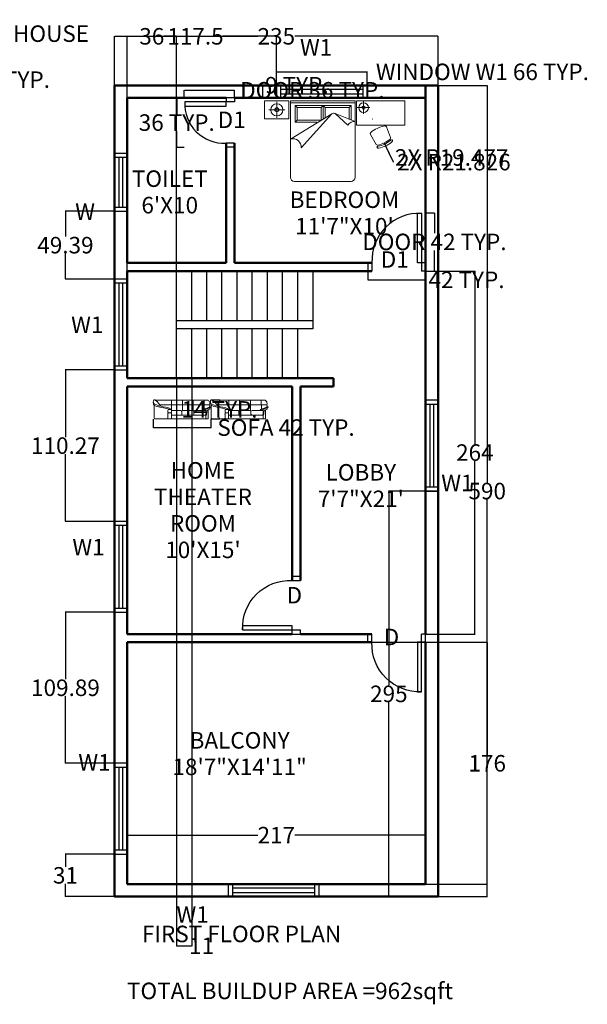
# Model space of a CAD drawing. Units: inches. Extents: x -15 to 810, y -55 to 662.
# Tile 3 of 3: x 397 to 810, y -55 to 662. Entities that reach past the tile are written whole.
import ezdxf
from ezdxf.enums import TextEntityAlignment as Align

# ---------------------------------------------------------------- set-up
doc = ezdxf.new("R2010")
doc.units = ezdxf.units.IN
doc.header["$MEASUREMENT"] = 0
for name, color, linetype, lineweight in [('A-ANNO-DIMS', 2, 'Continuous', 18), ('A-ANNO-TEXT', 1, 'Continuous', 25), ('A-AREA-IDEN', 1, 'Continuous', 25), ('A-DOOR', 2, 'Continuous', 25), ('A-FLOR-STRS', 3, 'Continuous', 25), ('A-FURN', 8, 'Continuous', 18), ('A-GLAZ', 4, 'Continuous', 18), ('A-WALL', 6, 'Continuous', 50)]:
    doc.layers.add(name, color=color, linetype=linetype, lineweight=lineweight)
doc.layers.add('Layer3', color=4, linetype='Continuous')
doc.styles.get("Standard").update_dxf_attribs({"font": 'arial.ttf'})
doc.dimstyles.get("Standard").update_dxf_attribs({"dimtxt": 12, "dimasz": 0.18, "dimexe": 0.18, "dimexo": 0.0625, "dimgap": 0.09, "dimtad": 0, "dimtih": 1, "dimtoh": 1, "dimdec": 0, "dimzin": 0, "dimdsep": 46, "dimlunit": 4, "dimtxsty": 'Standard', "dimcen": 0.09, "dimadec": 0, "dimazin": 0, "dimtfac": 1, "dimtdec": 0, "dimtofl": 0, "dimtmove": 0, "dimatfit": 3, "dimfxl": 1, "dimtolj": 1, "dimtzin": 0, "dimarcsym": 0})

# ---------------------------------------------------------------- blocks, each defined once
blk = doc.blocks.new('A$C21DD57CF')
for p, q in [((0, 682), (8, 763)), ((0, 682), (8, 763)), ((37, 628), (0, 682)), ((37, 628), (0, 682)), ((8, 763), (29, 794)), ((8, 763), (29, 794)), ((16, 616), (16, 655)), ((16, 616), (16, 655)), ((35, 572), (16, 616)), ((35, 572), (16, 616)), ((29, 794), (63, 792)), ((29, 794), (63, 792)), ((35, 574), (141, 516)), ((35, 574), (141, 516)), ((36, 32), (36, 574)), ((36, 32), (36, 574)), ((159, 572), (37, 631)), ((159, 572), (37, 631)), ((63, 792), (74, 786)), ((63, 792), (74, 786)), ((74, 786), (2250, 786)), ((74, 786), (173, 714)), ((74, 786), (2250, 786)), ((74, 786), (173, 714)), ((141, 516), (218, 501)), ((141, 516), (218, 501)), ((228, 550), (159, 572)), ((228, 550), (159, 572)), ((173, 714), (247, 611)), ((173, 714), (247, 611)), ((218, 501), (326, 479)), ((218, 501), (326, 479)), ((334, 528), (228, 550)), ((334, 528), (228, 550)), ((247, 611), (314, 530)), ((247, 611), (314, 530)), ((274, 586), (2345, 589)), ((274, 586), (2345, 589)), ((326, 479), (422, 460)), ((326, 479), (422, 460)), ((414, 506), (334, 528)), ((414, 506), (334, 528)), ((517, 484), (414, 506)), ((517, 484), (414, 506)), ((422, 460), (501, 445)), ((422, 460), (501, 445)), ((501, 445), (660, 413)), ((501, 445), (660, 413)), ((636, 460), (517, 484)), ((636, 460), (517, 484)), ((703, 430), (636, 460)), ((703, 430), (636, 460)), ((640, 786), (761, 786)), ((640, 786), (761, 786)), ((660, 413), (685, 398)), ((660, 413), (685, 398)), ((701, 430), (719, 398)), ((701, 430), (719, 398)), ((703, 427), (703, 430)), ((703, 427), (703, 430)), ((761, 786), (761, 356)), ((761, 786), (761, 356)), ((1211, 356), (1211, 786)), ((1211, 786), (1661, 786)), ((1211, 356), (1211, 786)), ((1211, 786), (1661, 786)), ((1661, 786), (1661, 347)), ((1661, 786), (1661, 347)), ((2346, 495), (2076, 394)), ((2346, 495), (2076, 394)), ((2082, 357), (2343, 458)), ((2082, 357), (2343, 458)), ((2116, 783), (2119, 410)), ((2116, 783), (2119, 410)), ((2343, 458), (2393, 477)), ((2343, 458), (2393, 477)), ((2356, 445), (2343, 458)), ((2356, 445), (2343, 458)), ((2346, 495), (2346, 509)), ((2346, 495), (2346, 509)), ((2346, 495), (2386, 508)), ((2346, 495), (2386, 508)), ((2354, 413), (2346, 403)), ((2354, 413), (2346, 403)), ((2356, 428), (2354, 413)), ((2356, 428), (2354, 413)), ((2356, 428), (2356, 445)), ((2356, 428), (2356, 445)), ((2394, 499), (2386, 508)), ((2394, 499), (2386, 508)), ((2393, 477), (2397, 489)), ((2393, 477), (2397, 489)), ((2397, 489), (2394, 499)), ((2397, 489), (2394, 499)), ((35, 34), (51, 7)), ((35, 34), (51, 7)), ((36, 32), (36, 400)), ((36, 32), (36, 400)), ((51, 7), (84, 0)), ((51, 7), (84, 0)), ((732, 0), (83, 0)), ((732, 0), (83, 0)), ((605, 205), (613, 235)), ((605, 205), (613, 235)), ((605, 27), (615, 10)), ((605, 27), (615, 10)), ((617, 384), (606, 354)), ((617, 384), (606, 354)), ((606, 294), (606, 354)), ((606, 294), (606, 354)), ((606, 294), (609, 276)), ((606, 294), (609, 276)), ((606, 25), (606, 208)), ((606, 25), (606, 208)), ((732, 0), (606, 0)), ((732, 0), (606, 0)), ((609, 276), (619, 264)), ((609, 276), (619, 264)), ((613, 235), (619, 244)), ((613, 235), (619, 244)), ((615, 10), (636, 0)), ((615, 10), (636, 0)), ((646, 398), (617, 384)), ((646, 398), (617, 384)), ((619, 264), (644, 249)), ((619, 264), (644, 249)), ((619, 244), (640, 249)), ((619, 244), (640, 249)), ((736, 250), (642, 250)), ((736, 250), (642, 250)), ((719, 398), (646, 398)), ((719, 398), (646, 398)), ((719, 398), (731, 398)), ((719, 398), (731, 398)), ((731, 398), (748, 389)), ((731, 398), (748, 389)), ((731, 0), (748, 10)), ((731, 0), (748, 10)), ((733, 249), (748, 244)), ((733, 249), (748, 244)), ((735, 249), (752, 264)), ((735, 249), (752, 264)), ((740, 5), (2289, 5)), ((740, 5), (2289, 5)), ((748, 389), (757, 371)), ((748, 389), (757, 371)), ((748, 244), (754, 233)), ((748, 244), (754, 233)), ((748, 10), (756, 27)), ((748, 10), (756, 27)), ((752, 264), (756, 287)), ((752, 264), (756, 287)), ((2131, 156), (752, 156)), ((2131, 156), (752, 156)), ((754, 233), (756, 24)), ((754, 233), (756, 24)), ((757, 371), (756, 287)), ((757, 371), (756, 287)), ((761, 356), (1134, 356)), ((761, 356), (1134, 356)), ((797, 356), (1134, 356)), ((797, 356), (1134, 356)), ((1134, 356), (1160, 345)), ((1134, 356), (1160, 345)), ((1152, 156), (1171, 160)), ((1152, 156), (1171, 160)), ((1160, 345), (1180, 324)), ((1160, 345), (1180, 324)), ((1171, 160), (1183, 174)), ((1171, 160), (1183, 174)), ((1180, 324), (1186, 313)), ((1180, 324), (1186, 313)), ((1183, 174), (1185, 192)), ((1183, 174), (1185, 192)), ((1185, 192), (1185, 315)), ((1185, 192), (1185, 315)), ((1185, 192), (1200, 160)), ((1185, 192), (1200, 160)), ((1200, 160), (1232, 156)), ((1200, 160), (1232, 156)), ((1225, 356), (1633, 356)), ((1225, 356), (1633, 356)), ((1633, 356), (1667, 345)), ((1633, 356), (1667, 345)), ((1676, 174), (1649, 154)), ((1676, 174), (1649, 154)), ((1667, 345), (1685, 326)), ((1667, 345), (1685, 326)), ((1687, 195), (1676, 174)), ((1687, 195), (1676, 174)), ((1684, 324), (1705, 338)), ((1684, 324), (1705, 338)), ((1684, 195), (1705, 164)), ((1684, 195), (1705, 164)), ((1685, 326), (1685, 159)), ((1685, 326), (1685, 159)), ((1705, 338), (1733, 356)), ((1705, 338), (1733, 356)), ((1705, 164), (1736, 154)), ((1705, 164), (1736, 154)), ((1733, 356), (2144, 356)), ((1733, 356), (2111, 356)), ((1733, 356), (2144, 356)), ((1733, 356), (2111, 356)), ((2076, 394), (2074, 374)), ((2076, 394), (2074, 374)), ((2074, 374), (2078, 364)), ((2074, 374), (2078, 364)), ((2078, 364), (2082, 357)), ((2078, 364), (2082, 357)), ((2119, 356), (2119, 371)), ((2119, 356), (2119, 371)), ((2170, 161), (2131, 156)), ((2170, 161), (2131, 156)), ((2144, 356), (2178, 351)), ((2144, 356), (2178, 351)), ((2191, 178), (2170, 161)), ((2191, 178), (2170, 161)), ((2178, 351), (2192, 333)), ((2178, 351), (2192, 333)), ((2194, 194), (2191, 178)), ((2194, 194), (2191, 178)), ((2192, 333), (2194, 320)), ((2192, 333), (2194, 320)), ((2194, 348), (2193, 348)), ((2194, 348), (2193, 348)), ((2194, 400), (2194, 5)), ((2194, 400), (2194, 5)), ((2210, 156), (2194, 156)), ((2210, 156), (2194, 156)), ((2218, 183), (2210, 156)), ((2218, 183), (2210, 156)), ((2225, 287), (2218, 183)), ((2225, 287), (2218, 183)), ((2242, 360), (2225, 287)), ((2242, 360), (2225, 287)), ((2286, 378), (2242, 360)), ((2286, 378), (2242, 360)), ((2346, 403), (2288, 378)), ((2346, 403), (2288, 378)), ((2288, 378), (2289, 5)), ((2288, 378), (2289, 5))]:
    blk.add_line(p, q)
for centre, radius, start, end in [((2206, 643), 150, 338.8976, 73.2177), ((2206, 643), 150, 338.8976, 73.2177), ((2286, 548), 72.2, 326.352, 34.4802), ((2286, 548), 72.2, 326.352, 34.4802), ((1228, 313), 43.2, 92.4362, 179.0526), ((1228, 313), 43.2, 92.4362, 179.0526)]:
    blk.add_arc(centre, radius, start, end)
blk = doc.blocks.new('A$C44EF7260')
for p, q in [((0, 1.998), (0.6, 1.998)), ((0, 1.548), (0, 1.998)), ((0.304, 1.579), (0.304, 1.971)), ((0.6, 1.998), (0.6, 1.548)), ((0.64, 2), (2.24, 2)), ((0.64, 0.1), (0.64, 2)), ((2.24, 2), (2.24, 0.1)), ((3.476, 1.998), (2.276, 1.998)), ((2.276, 1.998), (2.276, 1.398)), ((2.45, 1.671), (2.45, 1.985)), ((3.476, 1.398), (3.476, 1.998)), ((0.106, 1.775), (0.503, 1.775)), ((0.64, 1.95), (2.24, 1.95)), ((0.759, 1.884), (2.147, 1.884)), ((0.759, 1.884), (0.809, 1.834)), ((0.759, 1.467), (0.759, 1.884)), ((0.809, 1.834), (1.403, 1.834)), ((0.809, 1.517), (0.809, 1.834)), ((1.403, 1.834), (1.453, 1.884)), ((1.403, 1.834), (1.403, 1.53)), ((1.453, 1.884), (1.503, 1.834)), ((1.453, 1.884), (1.453, 1.558)), ((1.503, 1.834), (1.503, 1.586)), ((1.503, 1.834), (2.097, 1.834)), ((2.097, 1.834), (2.147, 1.884)), ((2.097, 1.834), (2.097, 1.535)), ((2.147, 1.884), (2.147, 1.519)), ((2.609, 1.828), (2.291, 1.828)), ((0.6, 1.548), (0, 1.548)), ((0.64, 1.05), (1.666, 1.676)), ((0.809, 1.517), (0.759, 1.467)), ((1.29, 1.467), (0.759, 1.467)), ((1.38, 1.517), (0.809, 1.517)), ((0.906, 0.833), (1.666, 1.676)), ((1.746, 1.684), (2.246, 1.486)), ((1.746, 1.684), (2.06, 1.397)), ((2.276, 1.398), (3.476, 1.398)), ((3.017, 1.352), (3.118, 1.091)), ((2.619, 1.162), (2.759, 0.919)), ((0.907, 0.845), (0.919, 0.845)), ((2.14, 0), (0.74, 0))]:
    blk.add_line(p, q)
for centre, radius in [((0.304, 1.775), 0.15), ((0.304, 1.775), 0.05), ((2.45, 1.828), 0.12), ((2.45, 1.828), 0.04)]:
    blk.add_circle(centre, radius)
for centre, radius, start, end in [((1.715, 1.589), 0.1, 71.7215, 119.0799), ((2.226, 1.289), 0.198, 84.1725, 146.9889), ((3.157, 0.547), 0.85, 102.6739, 128.3957), ((2.979, 1.337), 0.04, 21.3259, 102.6739), ((0.7, 0.852), 0.207, 354.6422, 106.9775), ((2.654, 1.182), 0.04, 128.3957, 209.9042), ((2.677, 1.551), 0.663, 280.7977, 310.4324), ((2.677, 1.551), 0.693, 280.6958, 310.5343), ((2.677, 1.551), 0.743, 281.5789, 309.6512), ((3.081, 1.077), 0.04, 310.4324, 21.3259), ((3.147, 1.002), 0.03, 70.2086, 130.5343), ((3.126, 1.01), 0.04, 309.6512, 20.6936), ((3.154, 1.02), 0.01, 20.6936, 70.2086), ((2.794, 0.939), 0.04, 209.9042, 280.7977), ((2.792, 0.847), 0.01, 161.0215, 210.5365), ((2.811, 0.841), 0.03, 100.6958, 161.0215), ((2.818, 0.862), 0.04, 210.5365, 281.5789), ((0.74, 0.1), 0.1, 180, 270), ((2.14, 0.1), 0.1, 270, 0)]:
    blk.add_arc(centre, radius, start, end)
blk = doc.blocks.new('v')
at = {"layer": 'Layer3'}
for p, q in [((0, 0), (0, -9)), ((39, 0), (3, 0)), ((3, 0), (3, -9)), ((39, -9), (39, 0)), ((42, -9), (42, 0)), ((39, -3), (3, -3)), ((3, -6), (39, -6)), ((3, -9), (39, -9))]:
    blk.add_line(p, q, dxfattribs=at)
blk = doc.blocks.new('gh')
at = {"layer": 'Layer3'}
for p, q in [((0, 0), (0, -9)), ((63, 0), (3, 0)), ((3, 0), (3, -9)), ((63, -9), (63, 0)), ((66, -9), (66, 0)), ((63, -3), (3, -3)), ((3, -6), (63, -6)), ((3, -9), (63, -9))]:
    blk.add_line(p, q, dxfattribs=at)
blk = doc.blocks.new('DOOR-SWING-30IN')
for p, q in [((36.04, 36), (30.04, 36)), ((30.04, 36), (30.04, 33)), ((36.04, 36), (36.04, 33)), ((36.04, 33), (30.04, 33)), ((36.04, 3), (30.04, 3)), ((36.04, 0), (30.04, 0))]:
    blk.add_line(p, q)
blk.add_lwpolyline([(30.04, 33), (0.04, 33), (0.04, 30), (30.04, 30)], close=True)
blk.add_arc((28.54, 31.5), 28.54, 176.98721, 273.01279)
blk = doc.blocks.new('DOOR-SWING-36IN')
for p, q in [((0, 6), (0, 0)), ((3, 6), (3, 0)), ((39, 6), (39, 0)), ((42, 6), (39, 6)), ((42, 0), (39, 0)), ((42, 6), (42, 0))]:
    blk.add_line(p, q)
blk.add_lwpolyline([(39, 6), (36, 6), (36, 42), (39, 42)], close=True)
blk.add_arc((37.5, 7.5), 34.53, 87.51045, 182.48955)
blk = doc.blocks.new('STAIR-HALF-TURN')
for p, q in [((0, 78), (135, 78)), ((0, 0), (0, 78)), ((36, 0), (36, 78)), ((47, 42), (47, 78)), ((58, 42), (58, 78)), ((69, 42), (69, 78)), ((80, 42), (80, 78)), ((91, 42), (91, 78)), ((102, 42), (102, 78)), ((113, 42), (113, 78)), ((124, 42), (124, 78)), ((135, 78), (135, 36)), ((36, 42), (135, 42)), ((135, 36), (36, 36)), ((47, 0), (47, 36)), ((58, 0), (58, 36)), ((69, 0), (69, 36)), ((80, 0), (80, 36)), ((91, 0), (91, 36)), ((102, 0), (102, 36)), ((113, 0), (113, 36)), ((124, 0), (124, 36)), ((124, 0), (0, 0))]:
    blk.add_line(p, q)
blk.add_lwpolyline([(124, 60, 0, 0, 0), (11.12, 60, 0, 0, 0), (11.12, 18.31, 0, 0, 0), (69, 18, 12, 0, 0), (102, 18, 0, 0, 0)], format="xyseb")
blk = doc.blocks.new('*D12')
at = {"layer": 'A-ANNO-DIMS', "color": 0, "lineweight": -2, "transparency": 16777216}
for p, q in [((583.81, 613.77), (583.81, 623.78)), ((583.99, 623.6), (649.63, 623.6)), ((649.81, 613.77), (649.81, 623.78)), ((649.81, 623.6), (649.99, 623.6))]:
    blk.add_line(p, q, dxfattribs=at)
at = {"layer": 'A-ANNO-DIMS', "color": 0, "transparency": 16777216}
for points in [[(583.99, 623.63), (583.99, 623.57), (583.81, 623.6)], [(649.63, 623.63), (649.63, 623.57), (649.81, 623.6)]]:
    blk.add_solid(points, dxfattribs=at)
at = {"layer": 'Defpoints', "color": 0, "transparency": 16777216}
for p in [(649.81, 623.6), (583.81, 613.7), (649.81, 613.7)]:
    blk.add_point(p, dxfattribs=at)
at = {"layer": 'A-ANNO-DIMS', "color": 0, "transparency": 16777216, "insert": (733.54, 623.6), "char_height": 12, "attachment_point": 5}
blk.add_mtext('\\A1;WINDOW W1 66 TYP.', dxfattribs=at)
blk = doc.blocks.new('*D13')
at = {"layer": 'A-ANNO-DIMS', "color": 0, "lineweight": -2, "transparency": 16777216}
for p, q in [((583.75, 613.7), (573.73, 613.7)), ((573.91, 613.7), (573.91, 613.88)), ((573.91, 613.88), (574.09, 613.88)), ((573.91, 604.88), (573.91, 613.52)), ((583.75, 604.7), (573.73, 604.7))]:
    blk.add_line(p, q, dxfattribs=at)
at = {"layer": 'A-ANNO-DIMS', "color": 0, "transparency": 16777216}
for points in [[(573.88, 613.52), (573.94, 613.52), (573.91, 613.7)], [(573.88, 604.88), (573.94, 604.88), (573.91, 604.7)]]:
    blk.add_solid(points, dxfattribs=at)
at = {"layer": 'Defpoints', "color": 0, "transparency": 16777216}
for p in [(573.91, 613.7), (583.81, 613.7), (583.81, 604.7)]:
    blk.add_point(p, dxfattribs=at)
at = {"layer": 'A-ANNO-DIMS', "color": 0, "transparency": 16777216, "insert": (598.73, 613.88), "char_height": 12, "attachment_point": 5}
blk.add_mtext('\\A1;9 TYP.', dxfattribs=at)
blk = doc.blocks.new('*D18')
at = {"layer": 'A-ANNO-DIMS', "color": 0, "lineweight": -2, "transparency": 16777216}
for p, q in [((151.13, 602.68), (151.13, 618.1)), ((151.31, 617.92), (252.98, 617.92)), ((253.16, 602.68), (253.16, 618.1)), ((253.16, 617.92), (253.34, 617.92))]:
    blk.add_line(p, q, dxfattribs=at)
at = {"layer": 'A-ANNO-DIMS', "color": 0, "transparency": 16777216}
for points in [[(151.31, 617.95), (151.31, 617.89), (151.13, 617.92)], [(252.98, 617.95), (252.98, 617.89), (253.16, 617.92)]]:
    blk.add_solid(points, dxfattribs=at)
at = {"layer": 'Defpoints', "color": 0, "transparency": 16777216}
for p in [(253.16, 617.92), (151.13, 602.62), (253.16, 602.62)]:
    blk.add_point(p, dxfattribs=at)
at = {"layer": 'A-ANNO-DIMS', "color": 0, "transparency": 16777216, "insert": (339.66, 617.92), "char_height": 12, "attachment_point": 5}
blk.add_mtext('\\A1;BED GROUP 102 TYP.', dxfattribs=at)
blk = doc.blocks.new('*D20')
at = {"layer": 'A-ANNO-DIMS', "color": 0, "lineweight": -2, "transparency": 16777216}
for p, q in [((494.36, 371.1), (494.36, 364.7)), ((536.23, 371.1), (536.23, 364.7)), ((494.54, 364.88), (536.05, 364.88)), ((536.23, 364.88), (536.41, 364.88))]:
    blk.add_line(p, q, dxfattribs=at)
at = {"layer": 'A-ANNO-DIMS', "color": 0, "transparency": 16777216}
for points in [[(494.54, 364.91), (494.54, 364.85), (494.36, 364.88)], [(536.05, 364.91), (536.05, 364.85), (536.23, 364.88)]]:
    blk.add_solid(points, dxfattribs=at)
at = {"layer": 'Defpoints', "color": 0, "transparency": 16777216}
for p in [(494.36, 371.16), (536.23, 371.16), (536.23, 364.88)]:
    blk.add_point(p, dxfattribs=at)
at = {"layer": 'A-ANNO-DIMS', "color": 0, "transparency": 16777216, "insert": (590.83, 364.88), "char_height": 12, "attachment_point": 5}
blk.add_mtext('\\A1;SOFA 42 TYP.', dxfattribs=at)
blk = doc.blocks.new('*D21')
at = {"layer": 'A-ANNO-DIMS', "color": 0, "lineweight": -2, "transparency": 16777216}
for p, q in [((536.3, 385.04), (542.69, 385.04)), ((542.51, 384.86), (542.51, 384.22)), ((536.3, 371.16), (542.69, 371.16)), ((542.51, 371.34), (542.51, 371.98))]:
    blk.add_line(p, q, dxfattribs=at)
at = {"layer": 'A-ANNO-DIMS', "color": 0, "transparency": 16777216}
for points in [[(542.48, 384.86), (542.54, 384.86), (542.51, 385.04)], [(542.48, 371.34), (542.54, 371.34), (542.51, 371.16)]]:
    blk.add_solid(points, dxfattribs=at)
at = {"layer": 'Defpoints', "color": 0, "transparency": 16777216}
for p in [(536.23, 385.04), (542.51, 385.04), (536.23, 371.16)]:
    blk.add_point(p, dxfattribs=at)
at = {"layer": 'A-ANNO-DIMS', "color": 0, "transparency": 16777216, "insert": (542.51, 378.1), "char_height": 12, "attachment_point": 5}
blk.add_mtext('\\A1;14 TYP.', dxfattribs=at)
blk = doc.blocks.new('*D24')
at = {"layer": 'A-ANNO-DIMS', "color": 0, "lineweight": -2, "transparency": 16777216}
for p, q in [((516.89, 604.77), (516.89, 610.35)), ((517.07, 610.17), (553.13, 610.17)), ((553.31, 604.77), (553.31, 610.35)), ((553.31, 610.17), (553.49, 610.17))]:
    blk.add_line(p, q, dxfattribs=at)
at = {"layer": 'A-ANNO-DIMS', "color": 0, "transparency": 16777216}
for points in [[(517.07, 610.2), (517.07, 610.14), (516.89, 610.17)], [(553.13, 610.2), (553.13, 610.14), (553.31, 610.17)]]:
    blk.add_solid(points, dxfattribs=at)
at = {"layer": 'Defpoints', "color": 0, "transparency": 16777216}
for p in [(553.31, 610.17), (516.89, 604.7), (553.31, 604.7)]:
    blk.add_point(p, dxfattribs=at)
at = {"layer": 'A-ANNO-DIMS', "color": 0, "transparency": 16777216, "insert": (609.97, 610.17), "char_height": 12, "attachment_point": 5}
blk.add_mtext('\\A1;DOOR 36 TYP.', dxfattribs=at)
blk = doc.blocks.new('*D25')
at = {"layer": 'A-ANNO-DIMS', "color": 0, "lineweight": -2, "transparency": 16777216}
for p, q in [((516.83, 604.7), (511.25, 604.7)), ((511.43, 604.52), (511.43, 592.92)), ((511.43, 568.88), (511.43, 580.48)), ((516.83, 568.7), (511.25, 568.7))]:
    blk.add_line(p, q, dxfattribs=at)
at = {"layer": 'A-ANNO-DIMS', "color": 0, "transparency": 16777216}
for points in [[(511.4, 604.52), (511.46, 604.52), (511.43, 604.7)], [(511.4, 568.88), (511.46, 568.88), (511.43, 568.7)]]:
    blk.add_solid(points, dxfattribs=at)
at = {"layer": 'Defpoints', "color": 0, "transparency": 16777216}
for p in [(511.43, 604.7), (516.89, 604.7), (516.89, 568.7)]:
    blk.add_point(p, dxfattribs=at)
at = {"layer": 'A-ANNO-DIMS', "color": 0, "transparency": 16777216, "insert": (511.43, 586.7), "char_height": 12, "attachment_point": 5}
blk.add_mtext('\\A1;36 TYP.', dxfattribs=at)
blk = doc.blocks.new('*D26')
at = {"layer": 'A-ANNO-DIMS', "color": 0, "lineweight": -2, "transparency": 16777216}
for p, q in [((692.38, 521.12), (698.86, 521.12)), ((698.68, 520.94), (698.68, 506.21)), ((698.68, 478.88), (698.68, 493.61)), ((692.38, 478.7), (698.86, 478.7))]:
    blk.add_line(p, q, dxfattribs=at)
at = {"layer": 'A-ANNO-DIMS', "color": 0, "transparency": 16777216}
for points in [[(698.65, 520.94), (698.71, 520.94), (698.68, 521.12)], [(698.65, 478.88), (698.71, 478.88), (698.68, 478.7)]]:
    blk.add_solid(points, dxfattribs=at)
at = {"layer": 'Defpoints', "color": 0, "transparency": 16777216}
for p in [(692.31, 521.12), (698.68, 521.12), (692.31, 478.7)]:
    blk.add_point(p, dxfattribs=at)
at = {"layer": 'A-ANNO-DIMS', "color": 0, "transparency": 16777216, "insert": (698.68, 499.91), "char_height": 12, "attachment_point": 5}
blk.add_mtext('\\A1;DOOR 42 TYP.', dxfattribs=at)
blk = doc.blocks.new('*D27')
at = {"layer": 'A-ANNO-DIMS', "color": 0, "lineweight": -2, "transparency": 16777216}
for p, q in [((650.31, 478.64), (650.31, 472.16)), ((692.31, 478.64), (692.31, 472.16)), ((650.49, 472.34), (692.13, 472.34)), ((692.31, 472.34), (692.49, 472.34))]:
    blk.add_line(p, q, dxfattribs=at)
at = {"layer": 'A-ANNO-DIMS', "color": 0, "transparency": 16777216}
for points in [[(650.49, 472.37), (650.49, 472.31), (650.31, 472.34)], [(692.13, 472.37), (692.13, 472.31), (692.31, 472.34)]]:
    blk.add_solid(points, dxfattribs=at)
at = {"layer": 'Defpoints', "color": 0, "transparency": 16777216}
for p in [(650.31, 478.7), (692.31, 478.7), (692.31, 472.34)]:
    blk.add_point(p, dxfattribs=at)
at = {"layer": 'A-ANNO-DIMS', "color": 0, "transparency": 16777216, "insert": (722.03, 472.34), "char_height": 12, "attachment_point": 5}
blk.add_mtext('\\A1;42 TYP.', dxfattribs=at)
blk = doc.blocks.new('*D36')
at = {"layer": 'A-ANNO-DIMS', "color": 0, "lineweight": -2, "transparency": 16777216}
for p, q in [((466.31, 613.77), (466.31, 649.63)), ((466.49, 649.45), (570.32, 649.45)), ((701.13, 649.45), (597.31, 649.45)), ((701.31, 613.77), (701.31, 649.63))]:
    blk.add_line(p, q, dxfattribs=at)
at = {"layer": 'A-ANNO-DIMS', "color": 0, "transparency": 16777216}
for points in [[(466.49, 649.48), (466.49, 649.42), (466.31, 649.45)], [(701.13, 649.48), (701.13, 649.42), (701.31, 649.45)]]:
    blk.add_solid(points, dxfattribs=at)
at = {"layer": 'Defpoints', "color": 0, "transparency": 16777216}
for p in [(701.31, 649.45), (466.31, 613.7), (701.31, 613.7)]:
    blk.add_point(p, dxfattribs=at)
at = {"layer": 'A-ANNO-DIMS', "color": 0, "transparency": 16777216, "insert": (583.81, 649.45), "char_height": 12, "attachment_point": 5}
blk.add_mtext('\\A1;235', dxfattribs=at)
blk = doc.blocks.new('*D37')
at = {"layer": 'A-ANNO-DIMS', "color": 0, "lineweight": -2, "transparency": 16777216}
for p, q in [((701.38, 613.7), (737.24, 613.7)), ((737.06, 613.52), (737.06, 324.92)), ((737.06, 23.88), (737.06, 312.49)), ((701.38, 23.7), (737.24, 23.7))]:
    blk.add_line(p, q, dxfattribs=at)
at = {"layer": 'A-ANNO-DIMS', "color": 0, "transparency": 16777216}
for points in [[(737.03, 613.52), (737.09, 613.52), (737.06, 613.7)], [(737.03, 23.88), (737.09, 23.88), (737.06, 23.7)]]:
    blk.add_solid(points, dxfattribs=at)
at = {"layer": 'Defpoints', "color": 0, "transparency": 16777216}
for p in [(701.31, 613.7), (737.06, 613.7), (701.31, 23.7)]:
    blk.add_point(p, dxfattribs=at)
at = {"layer": 'A-ANNO-DIMS', "color": 0, "transparency": 16777216, "insert": (737.06, 318.7), "char_height": 12, "attachment_point": 5}
blk.add_mtext('\\A1;590', dxfattribs=at)
blk = doc.blocks.new('*D42')
at = {"layer": 'A-ANNO-DIMS', "color": 0, "lineweight": -2, "transparency": 16777216}
for p, q in [((701.25, 318.7), (665.38, 318.7)), ((665.56, 318.52), (665.56, 177.42)), ((665.56, 23.88), (665.56, 164.99)), ((701.25, 23.7), (665.38, 23.7))]:
    blk.add_line(p, q, dxfattribs=at)
at = {"layer": 'A-ANNO-DIMS', "color": 0, "transparency": 16777216}
for points in [[(665.53, 318.52), (665.59, 318.52), (665.56, 318.7)], [(665.53, 23.88), (665.59, 23.88), (665.56, 23.7)]]:
    blk.add_solid(points, dxfattribs=at)
at = {"layer": 'Defpoints', "color": 0, "transparency": 16777216}
for p in [(665.56, 318.7), (701.31, 318.7), (701.31, 23.7)]:
    blk.add_point(p, dxfattribs=at)
at = {"layer": 'A-ANNO-DIMS', "color": 0, "transparency": 16777216, "insert": (665.56, 171.2), "char_height": 12, "attachment_point": 5}
blk.add_mtext('\\A1;295', dxfattribs=at)
blk = doc.blocks.new('*D43')
at = {"layer": 'A-ANNO-DIMS', "color": 0, "lineweight": -2, "transparency": 16777216}
for p, q in [((466.25, 54.7), (430.38, 54.7)), ((430.56, 54.52), (430.56, 45.42)), ((430.56, 23.88), (430.56, 32.98)), ((466.25, 23.7), (430.38, 23.7))]:
    blk.add_line(p, q, dxfattribs=at)
at = {"layer": 'A-ANNO-DIMS', "color": 0, "transparency": 16777216}
for points in [[(430.53, 54.52), (430.59, 54.52), (430.56, 54.7)], [(430.53, 23.88), (430.59, 23.88), (430.56, 23.7)]]:
    blk.add_solid(points, dxfattribs=at)
at = {"layer": 'Defpoints', "color": 0, "transparency": 16777216}
for p in [(430.56, 54.7), (466.31, 54.7), (466.31, 23.7)]:
    blk.add_point(p, dxfattribs=at)
at = {"layer": 'A-ANNO-DIMS', "color": 0, "transparency": 16777216, "insert": (430.56, 39.2), "char_height": 12, "attachment_point": 5}
blk.add_mtext('\\A1;31', dxfattribs=at)
blk = doc.blocks.new('*D44')
at = {"layer": 'A-ANNO-DIMS', "color": 0, "lineweight": -2, "transparency": 16777216}
for p, q in [((466.25, 230.59), (430.38, 230.59)), ((430.56, 230.41), (430.56, 181.86)), ((430.56, 120.88), (430.56, 169.43)), ((466.25, 120.7), (430.38, 120.7))]:
    blk.add_line(p, q, dxfattribs=at)
at = {"layer": 'A-ANNO-DIMS', "color": 0, "transparency": 16777216}
for points in [[(430.53, 230.41), (430.59, 230.41), (430.56, 230.59)], [(430.53, 120.88), (430.59, 120.88), (430.56, 120.7)]]:
    blk.add_solid(points, dxfattribs=at)
at = {"layer": 'Defpoints', "color": 0, "transparency": 16777216}
for p in [(430.56, 230.59), (466.31, 230.59), (466.31, 120.7)]:
    blk.add_point(p, dxfattribs=at)
at = {"layer": 'A-ANNO-DIMS', "color": 0, "transparency": 16777216, "insert": (430.56, 175.65), "char_height": 12, "attachment_point": 5}
blk.add_mtext('\\A1;109.89', dxfattribs=at)
blk = doc.blocks.new('*D45')
at = {"layer": 'A-ANNO-DIMS', "color": 0, "lineweight": -2, "transparency": 16777216}
for p, q in [((466.25, 406.86), (430.38, 406.86)), ((430.56, 406.68), (430.56, 357.94)), ((430.56, 296.77), (430.56, 345.51)), ((466.25, 296.59), (430.38, 296.59))]:
    blk.add_line(p, q, dxfattribs=at)
at = {"layer": 'A-ANNO-DIMS', "color": 0, "transparency": 16777216}
for points in [[(430.53, 406.68), (430.59, 406.68), (430.56, 406.86)], [(430.53, 296.77), (430.59, 296.77), (430.56, 296.59)]]:
    blk.add_solid(points, dxfattribs=at)
at = {"layer": 'Defpoints', "color": 0, "transparency": 16777216}
for p in [(430.56, 406.86), (466.31, 406.86), (466.31, 296.59)]:
    blk.add_point(p, dxfattribs=at)
at = {"layer": 'A-ANNO-DIMS', "color": 0, "transparency": 16777216, "insert": (430.56, 351.72), "char_height": 12, "attachment_point": 5}
blk.add_mtext('\\A1;110.27', dxfattribs=at)
blk = doc.blocks.new('*D46')
at = {"layer": 'A-ANNO-DIMS', "color": 0, "lineweight": -2, "transparency": 16777216}
for p, q in [((466.25, 522.24), (430.38, 522.24)), ((430.56, 522.06), (430.56, 503.77)), ((430.56, 473.04), (430.56, 491.33)), ((466.25, 472.86), (430.38, 472.86))]:
    blk.add_line(p, q, dxfattribs=at)
at = {"layer": 'A-ANNO-DIMS', "color": 0, "transparency": 16777216}
for points in [[(430.53, 522.06), (430.59, 522.06), (430.56, 522.24)], [(430.53, 473.04), (430.59, 473.04), (430.56, 472.86)]]:
    blk.add_solid(points, dxfattribs=at)
at = {"layer": 'Defpoints', "color": 0, "transparency": 16777216}
for p in [(430.56, 522.24), (466.31, 522.24), (466.31, 472.86)]:
    blk.add_point(p, dxfattribs=at)
at = {"layer": 'A-ANNO-DIMS', "color": 0, "transparency": 16777216, "insert": (430.56, 497.55), "char_height": 12, "attachment_point": 5}
blk.add_mtext('\\A1;49.39', dxfattribs=at)
blk = doc.blocks.new('*D47')
at = {"layer": 'A-ANNO-DIMS', "color": 0, "lineweight": -2, "transparency": 16777216}
for p, q in [((466.31, 613.77), (466.31, 649.63)), ((466.49, 649.45), (505.25, 649.45)), ((583.63, 649.45), (544.88, 649.45)), ((583.81, 613.77), (583.81, 649.63))]:
    blk.add_line(p, q, dxfattribs=at)
at = {"layer": 'A-ANNO-DIMS', "color": 0, "transparency": 16777216}
for points in [[(466.49, 649.48), (466.49, 649.42), (466.31, 649.45)], [(583.63, 649.48), (583.63, 649.42), (583.81, 649.45)]]:
    blk.add_solid(points, dxfattribs=at)
at = {"layer": 'Defpoints', "color": 0, "transparency": 16777216}
for p in [(466.31, 649.45), (466.31, 613.7), (583.81, 613.7)]:
    blk.add_point(p, dxfattribs=at)
at = {"layer": 'A-ANNO-DIMS', "color": 0, "transparency": 16777216, "insert": (525.06, 649.45), "char_height": 12, "attachment_point": 5}
blk.add_mtext('\\A1;117.5', dxfattribs=at)
blk = doc.blocks.new('*D48')
at = {"layer": 'A-ANNO-DIMS', "color": 0, "lineweight": -2, "transparency": 16777216}
for p, q in [((475.38, 208.7), (737.24, 208.7)), ((737.06, 208.52), (737.06, 126.92)), ((737.06, 32.88), (737.06, 114.49)), ((475.38, 32.7), (737.24, 32.7))]:
    blk.add_line(p, q, dxfattribs=at)
at = {"layer": 'A-ANNO-DIMS', "color": 0, "transparency": 16777216}
for points in [[(737.03, 208.52), (737.09, 208.52), (737.06, 208.7)], [(737.03, 32.88), (737.09, 32.88), (737.06, 32.7)]]:
    blk.add_solid(points, dxfattribs=at)
at = {"layer": 'Defpoints', "color": 0, "transparency": 16777216}
for p in [(475.31, 208.7), (737.06, 208.7), (475.31, 32.7)]:
    blk.add_point(p, dxfattribs=at)
at = {"layer": 'A-ANNO-DIMS', "color": 0, "transparency": 16777216, "insert": (737.06, 120.7), "char_height": 12, "attachment_point": 5}
blk.add_mtext('\\A1;176', dxfattribs=at)
blk = doc.blocks.new('*D49')
at = {"layer": 'A-ANNO-DIMS', "color": 0, "lineweight": -2, "transparency": 16777216}
for p, q in [((475.31, 32.77), (475.31, 68.63)), ((475.49, 68.45), (570.37, 68.45)), ((692.13, 68.45), (597.26, 68.45)), ((692.31, 32.77), (692.31, 68.63))]:
    blk.add_line(p, q, dxfattribs=at)
at = {"layer": 'A-ANNO-DIMS', "color": 0, "transparency": 16777216}
for points in [[(475.49, 68.48), (475.49, 68.42), (475.31, 68.45)], [(692.13, 68.48), (692.13, 68.42), (692.31, 68.45)]]:
    blk.add_solid(points, dxfattribs=at)
at = {"layer": 'Defpoints', "color": 0, "transparency": 16777216}
for p in [(692.31, 68.45), (475.31, 32.7), (692.31, 32.7)]:
    blk.add_point(p, dxfattribs=at)
at = {"layer": 'A-ANNO-DIMS', "color": 0, "transparency": 16777216, "insert": (583.81, 68.45), "char_height": 12, "attachment_point": 5}
blk.add_mtext('\\A1;217', dxfattribs=at)
blk = doc.blocks.new('*D53')
at = {"layer": 'A-ANNO-DIMS', "color": 0, "lineweight": -2, "transparency": 16777216}
for p, q in [((475.31, 400.77), (475.31, 649.63)), ((475.49, 649.45), (484.64, 649.45)), ((511.13, 649.45), (501.99, 649.45)), ((511.31, 400.77), (511.31, 649.63))]:
    blk.add_line(p, q, dxfattribs=at)
at = {"layer": 'A-ANNO-DIMS', "color": 0, "transparency": 16777216}
for points in [[(475.49, 649.48), (475.49, 649.42), (475.31, 649.45)], [(511.13, 649.48), (511.13, 649.42), (511.31, 649.45)]]:
    blk.add_solid(points, dxfattribs=at)
at = {"layer": 'Defpoints', "color": 0, "transparency": 16777216}
for p in [(511.31, 649.45), (475.31, 400.7), (511.31, 400.7)]:
    blk.add_point(p, dxfattribs=at)
at = {"layer": 'A-ANNO-DIMS', "color": 0, "transparency": 16777216, "insert": (493.31, 649.45), "char_height": 12, "attachment_point": 5}
blk.add_mtext('\\A1;36', dxfattribs=at)
blk = doc.blocks.new('*D54')
at = {"layer": 'A-ANNO-DIMS', "color": 0, "lineweight": -2, "transparency": 16777216}
for p, q in [((511.31, 400.64), (511.31, -12.23)), ((522.31, 400.64), (522.31, -12.23)), ((511.49, -12.05), (522.13, -12.05)), ((522.31, -12.05), (522.49, -12.05))]:
    blk.add_line(p, q, dxfattribs=at)
at = {"layer": 'A-ANNO-DIMS', "color": 0, "transparency": 16777216}
for points in [[(511.49, -12.02), (511.49, -12.08), (511.31, -12.05)], [(522.13, -12.02), (522.13, -12.08), (522.31, -12.05)]]:
    blk.add_solid(points, dxfattribs=at)
at = {"layer": 'Defpoints', "color": 0, "transparency": 16777216}
for p in [(511.31, 400.7), (522.31, 400.7), (522.31, -12.05)]:
    blk.add_point(p, dxfattribs=at)
at = {"layer": 'A-ANNO-DIMS', "color": 0, "transparency": 16777216, "insert": (529.46, -12.05), "char_height": 12, "attachment_point": 5}
blk.add_mtext('\\A1;11', dxfattribs=at)
blk = doc.blocks.new('*D55')
at = {"layer": 'A-ANNO-DIMS', "color": 0, "lineweight": -2, "transparency": 16777216}
for p, q in [((692.38, 478.7), (728.24, 478.7)), ((728.06, 478.52), (728.06, 352.92)), ((728.06, 214.88), (728.06, 340.49)), ((692.38, 214.7), (728.24, 214.7))]:
    blk.add_line(p, q, dxfattribs=at)
at = {"layer": 'A-ANNO-DIMS', "color": 0, "transparency": 16777216}
for points in [[(728.03, 478.52), (728.09, 478.52), (728.06, 478.7)], [(728.03, 214.88), (728.09, 214.88), (728.06, 214.7)]]:
    blk.add_solid(points, dxfattribs=at)
at = {"layer": 'Defpoints', "color": 0, "transparency": 16777216}
for p in [(692.31, 478.7), (692.31, 214.7), (728.06, 214.7)]:
    blk.add_point(p, dxfattribs=at)
at = {"layer": 'A-ANNO-DIMS', "color": 0, "transparency": 16777216, "insert": (728.06, 346.7), "char_height": 12, "attachment_point": 5}
blk.add_mtext('\\A1;264', dxfattribs=at)
blk = doc.blocks.new('*D60')
at = {"layer": 'A-ANNO-DIMS', "color": 0, "lineweight": -2, "transparency": 16777216}
for p, q in [((653.75, 589.45), (653.93, 589.45)), ((653.84, 589.36), (653.84, 589.54)), ((668.93, 557.96), (663.35, 569.6)), ((669.11, 557.96), (668.93, 557.96))]:
    blk.add_line(p, q, dxfattribs=at)
at = {"layer": 'A-ANNO-DIMS', "color": 0, "transparency": 16777216}
blk.add_solid([(663.38, 569.62), (663.32, 569.59), (663.27, 569.77)], dxfattribs=at)
at = {"layer": 'Defpoints', "color": 0, "transparency": 16777216}
for p in [(653.84, 589.45), (663.27, 569.77)]:
    blk.add_point(p, dxfattribs=at)
at = {"layer": 'A-ANNO-DIMS', "color": 0, "transparency": 16777216, "insert": (712.84, 557.96), "char_height": 12, "attachment_point": 5}
blk.add_mtext('\\A1;2X R21.826', dxfattribs=at)
blk = doc.blocks.new('*D62')
at = {"layer": 'A-ANNO-DIMS', "color": 0, "lineweight": -2, "transparency": 16777216}
for p, q in [((653.75, 589.45), (653.93, 589.45)), ((653.84, 589.36), (653.84, 589.54)), ((667.31, 561.35), (662.33, 571.72)), ((667.49, 561.35), (667.31, 561.35))]:
    blk.add_line(p, q, dxfattribs=at)
at = {"layer": 'A-ANNO-DIMS', "color": 0, "transparency": 16777216}
blk.add_solid([(662.36, 571.73), (662.31, 571.71), (662.26, 571.88)], dxfattribs=at)
at = {"layer": 'Defpoints', "color": 0, "transparency": 16777216}
for p in [(653.84, 589.45), (662.26, 571.88)]:
    blk.add_point(p, dxfattribs=at)
at = {"layer": 'A-ANNO-DIMS', "color": 0, "transparency": 16777216, "insert": (711.22, 561.35), "char_height": 12, "attachment_point": 5}
blk.add_mtext('\\A1;2X R19.477', dxfattribs=at)

msp = doc.modelspace()

# ---------------------------------------------------------------- linework, layer by layer
at = {"layer": 'A-WALL'}
for p, q in [((692.3149, 214.7034), (692.3149, 613.7034)), ((547.3149, 604.7034), (475.3149, 604.7034)), ((475.3149, 604.7034), (475.3149, 484.7034)), ((692.3149, 604.7034), (553.3149, 604.7034)), ((692.3149, 484.7034), (692.3149, 604.7034)), ((547.3149, 571.7034), (547.3149, 484.7034)), ((553.3149, 571.7034), (553.3149, 484.7034)), ((547.3149, 484.7034), (475.3149, 484.7034)), ((653.3149, 484.7034), (553.3149, 484.7034)), ((653.3149, 478.7034), (475.3149, 478.7034)), ((475.3149, 478.7034), (475.3149, 400.7034)), ((692.3149, 214.7034), (692.3149, 478.7034)), ((475.3149, 400.7034), (625.3149, 400.7034)), ((475.3149, 394.7034), (595.3149, 394.7034)), ((475.3149, 394.7034), (475.3149, 214.7034)), ((595.3149, 394.7034), (595.3149, 253.7034)), ((601.3149, 394.7034), (625.3149, 394.7034)), ((601.3149, 394.7034), (601.3149, 253.7034)), ((625.3149, 394.7034), (625.3149, 400.7034)), ((475.3149, 214.7034), (595.3149, 214.7034)), ((475.3149, 208.7034), (653.3149, 208.7034)), ((475.3149, 208.7034), (475.3149, 32.7034)), ((601.3149, 214.7034), (653.3149, 214.7034)), ((601.3149, 214.7034), (625.3149, 214.7034)), ((692.3149, 32.7034), (692.3149, 208.7034)), ((475.3149, 32.7034), (692.3149, 32.7034)), ((689.3149, 32.7034), (692.3149, 32.7034))]:
    msp.add_line(p, q, dxfattribs=at)
msp.add_lwpolyline([(689.3149, 23.7034), (701.3149, 23.7034), (701.3149, 613.7034), (466.3149, 613.7034), (466.3149, 23.7034), (701.3149, 23.7034)], dxfattribs=at)

# ---------------------------------------------------------------- block references
at = {"layer": 'A-DOOR'}
for name, p in [('DOOR-SWING-30IN', (517.2757, 568.703)), ('DOOR-SWING-36IN', (650.3147, 478.703))]:
    msp.add_blockref(name, p, dxfattribs=at)
at = {"layer": 'A-DOOR', "extrusion": (0, 0, -1), "zscale": -1}
for p, rotation in [((-601.3153, 256.7036), 269.9999999999999), ((-650.3147, 214.7039), 180)]:
    msp.add_blockref('DOOR-SWING-36IN', p, dxfattribs=dict(at, rotation=rotation))
at = {"layer": 'A-FLOR-STRS'}
msp.add_blockref('STAIR-HALF-TURN', (475.3147, 400.703), dxfattribs=at)
at = {"layer": 'A-FURN'}
for name, p, xscale, yscale, zscale in [('A$C44EF7260', (575.2545, 543.9012), 29.35705846695051, 29.35705846695051, 29.35705846695051), ('A$C21DD57CF', (494.3644, 371.1603), 0.0174704312386394, 0.0174704312386394, 0.0174704312386394), ('A$C21DD57CF', (535.9249, 371.1603), 0.0174704312386394, 0.0174704312386394, 0.0174704312386394)]:
    msp.add_blockref(name, p, dxfattribs=dict(at, xscale=xscale, yscale=yscale, zscale=zscale))
at = {"layer": 'A-GLAZ'}
for p in [(583.8149, 613.7034), (548.903, 32.804)]:
    msp.add_blockref('gh', p, dxfattribs=at)
at = {"layer": 'A-GLAZ', "rotation": 90}
for name, p in [('v', (466.3149, 522.244)), ('gh', (466.3149, 406.8559)), ('gh', (692.3149, 318.7034)), ('gh', (466.3149, 230.5885)), ('gh', (466.3149, 54.7034))]:
    msp.add_blockref(name, p, dxfattribs=at)

# ---------------------------------------------------------------- texts
at = {"layer": 'A-ANNO-TEXT'}
for s, p in [('NORTH FACING HOUSE', (359.6923, 645.3791)), ('W1', (612.7052, 635.4492)), ('D1', (551.3492, 582.6817)), ('W', (444.8226, 515.8777)), ('D1', (669.8574, 481.1314)), ('W1', (446.4157, 433.6508)), ('W1', (715.3721, 318.6196)), ('W1', (447.3233, 271.9128)), ('D', (596.8878, 236.9364)), ('D', (667.4664, 206.5679)), ('W1', (451.6618, 115.3676)), ('W1', (522.9865, 4.6786)), ('FIRST FLOOR PLAN', (558.5444, -9.4261))]:
    msp.add_text(s, height=12, dxfattribs=at).set_placement(p, align=Align.CENTER)
at = {"layer": 'A-AREA-IDEN'}
for s, p in [('TOILET', (506.3675, 539.9157)), ("6'X10", (506.3675, 520.6388)), ('BEDROOM', (633.2959, 524.6153)), ('11\'7"X10\'', (633.2959, 505.3384)), ('HOME', (530.49, 327.7602)), ('LOBBY', (645.2092, 326.325)), ('THEATER', (530.49, 308.4832)), ('7\'7"X21\'', (645.2092, 307.0481)), ('ROOM', (530.49, 289.2063)), ("10'X15'", (530.49, 269.9293)), ('BALCONY', (557.1276, 131.3917)), ('18\'7"X14\'11"', (557.1276, 112.1148)), ('TOTAL BUILDUP AREA =962sqft', (593.7082, -50.8463))]:
    msp.add_text(s, height=12, dxfattribs=at).set_placement(p, align=Align.CENTER)

# ---------------------------------------------------------------- dimensions: what is measured, and where the dimension line sits
at = {"layer": 'A-ANNO-DIMS'}
for base, p1, p2, text, picture, middle in [((649.8149, 623.6034), (583.8149, 613.7034), (649.8149, 613.7034), 'WINDOW W1 <> TYP.', '*D12', (733.5446, 623.6034)), ((253.1593, 617.9222), (151.1262, 602.6172), (253.1593, 602.6172), 'BED GROUP <> TYP.', '*D18', (339.6599, 617.9222)), ((553.3149, 610.1672), (516.8897, 604.7034), (553.3149, 604.7034), 'DOOR <> TYP.', '*D24', (609.9669, 610.1672)), ((692.3149, 472.3404), (650.3149, 478.7034), (692.3149, 478.7034), '<> TYP.', '*D27', (722.0324, 472.3404)), ((536.2325, 364.8801), (494.3644, 371.1603), (536.2325, 371.1603), 'SOFA <> TYP.', '*D20', (590.8299, 364.8801))]:
    dim = msp.add_linear_dim(base=base, p1=p1, p2=p2, text=text, dimstyle='Standard', override={"dimdec": 0, "dimlfac": 1, "dimrnd": 0, "dimzin": 0, "dimdsep": 46, "dimlunit": 2}, dxfattribs=at)
    dim.commit()
    dim.dimension.update_dxf_attribs({"geometry": picture, "text_midpoint": middle})
for base, p1, p2, override, picture, middle in [((701.3149, 649.4534), (466.3149, 613.7034), (701.3149, 613.7034), {"dimdec": 0, "dimlfac": 1, "dimrnd": 0, "dimzin": 0, "dimdsep": 46, "dimlunit": 2}, '*D36', (583.8149, 649.4534)), ((466.3149, 649.4534), (583.8149, 613.7034), (466.3149, 613.7034), {"dimdec": 1, "dimlfac": 1, "dimrnd": 0, "dimzin": 0, "dimdsep": 46, "dimlunit": 2}, '*D47', (525.0649, 649.4534)), ((511.3149, 649.4534), (475.3149, 400.7034), (511.3149, 400.7034), {"dimdec": 0, "dimlfac": 1, "dimrnd": 0, "dimzin": 0, "dimdsep": 46, "dimlunit": 2}, '*D53', (493.3149, 649.4534)), ((522.3149, -12.0466), (511.3149, 400.7034), (522.3149, 400.7034), {"dimdec": 0, "dimlfac": 1, "dimrnd": 0, "dimzin": 0, "dimdsep": 46, "dimlunit": 2}, '*D54', (529.4566, -12.0466)), ((692.3149, 68.4534), (475.3149, 32.7034), (692.3149, 32.7034), {"dimdec": 0, "dimlfac": 1, "dimrnd": 0, "dimzin": 0, "dimdsep": 46, "dimlunit": 2}, '*D49', (583.8149, 68.4534))]:
    dim = msp.add_linear_dim(base=base, p1=p1, p2=p2, dimstyle='Standard', override=override, dxfattribs=at)
    dim.commit()
    dim.dimension.update_dxf_attribs({"geometry": picture, "text_midpoint": middle})
for base, p1, p2, text, picture, middle in [((573.9149, 613.7034), (583.8149, 604.7034), (583.8149, 613.7034), '<> TYP.', '*D13', (598.7292, 613.8834)), ((511.4259, 604.7034), (516.8897, 568.7034), (516.8897, 604.7034), '<> TYP.', '*D25', (511.4259, 586.7034)), ((698.678, 521.1239), (692.3149, 478.7034), (692.3149, 521.1239), 'DOOR <> TYP.', '*D26', (698.678, 499.9137)), ((542.5127, 385.0402), (536.2325, 371.1603), (536.2325, 385.0402), '<> TYP.', '*D21', (542.5127, 378.1002))]:
    dim = msp.add_linear_dim(base=base, p1=p1, p2=p2, angle=90, text=text, dimstyle='Standard', override={"dimdec": 0, "dimlfac": 1, "dimrnd": 0, "dimzin": 0, "dimdsep": 46, "dimlunit": 2}, dxfattribs=at)
    dim.commit()
    dim.dimension.update_dxf_attribs({"geometry": picture, "text_midpoint": middle})
for base, p1, p2, angle, override, picture, middle in [((737.0649, 613.7034), (701.3149, 23.7034), (701.3149, 613.7034), 90, {"dimdec": 0, "dimlfac": 1, "dimrnd": 0, "dimzin": 0, "dimdsep": 46, "dimlunit": 2}, '*D37', (737.0649, 318.7034)), ((430.5649, 522.244), (466.3149, 472.8559), (466.3149, 522.244), 90, {"dimdec": 2, "dimlfac": 1, "dimrnd": 0, "dimzin": 0, "dimdsep": 46, "dimlunit": 2}, '*D46', (430.5649, 497.55)), ((728.0649, 214.7034), (692.3149, 478.7034), (692.3149, 214.7034), 270, {"dimdec": 0, "dimlfac": 1, "dimrnd": 0, "dimzin": 0, "dimdsep": 46, "dimlunit": 2}, '*D55', (728.0649, 346.7034)), ((430.5649, 406.8559), (466.3149, 296.5885), (466.3149, 406.8559), 90, {"dimdec": 2, "dimlfac": 1, "dimrnd": 0, "dimzin": 0, "dimdsep": 46, "dimlunit": 2}, '*D45', (430.5649, 351.7222)), ((665.5649, 318.7034), (701.3149, 23.7034), (701.3149, 318.7034), 90, {"dimdec": 0, "dimlfac": 1, "dimrnd": 0, "dimzin": 0, "dimdsep": 46, "dimlunit": 2}, '*D42', (665.5649, 171.2034)), ((430.5649, 230.5885), (466.3149, 120.7034), (466.3149, 230.5885), 90, {"dimdec": 2, "dimlfac": 1, "dimrnd": 0, "dimzin": 0, "dimdsep": 46, "dimlunit": 2}, '*D44', (430.5649, 175.6459)), ((737.0649, 208.7034), (475.3149, 32.7034), (475.3149, 208.7034), 90, {"dimdec": 0, "dimlfac": 1, "dimrnd": 0, "dimzin": 0, "dimdsep": 46, "dimlunit": 2}, '*D48', (737.0649, 120.7034)), ((430.5649, 54.7034), (466.3149, 23.7034), (466.3149, 54.7034), 90, {"dimdec": 0, "dimlfac": 1, "dimrnd": 0, "dimzin": 0, "dimdsep": 46, "dimlunit": 2}, '*D43', (430.5649, 39.2034))]:
    dim = msp.add_linear_dim(base=base, p1=p1, p2=p2, angle=angle, dimstyle='Standard', override=override, dxfattribs=at)
    dim.commit()
    dim.dimension.update_dxf_attribs({"geometry": picture, "text_midpoint": middle})
for mpoint, picture, middle in [((663.2718, 569.7653), '*D60', (712.8444, 557.9568)), ((662.2569, 571.8832), '*D62', (711.2246, 561.3455))]:
    dim = msp.add_radius_dim(center=(653.8362, 589.4461), mpoint=mpoint, text='2X <>', dimstyle='Standard', override={"dimdec": 3, "dimlfac": 1, "dimrnd": 0, "dimzin": 0, "dimdsep": 46, "dimlunit": 2}, dxfattribs=at)
    dim.commit()
    dim.dimension.update_dxf_attribs({"geometry": picture, "text_midpoint": middle, "dimtype": 164})

doc.saveas('drawing.dxf')
